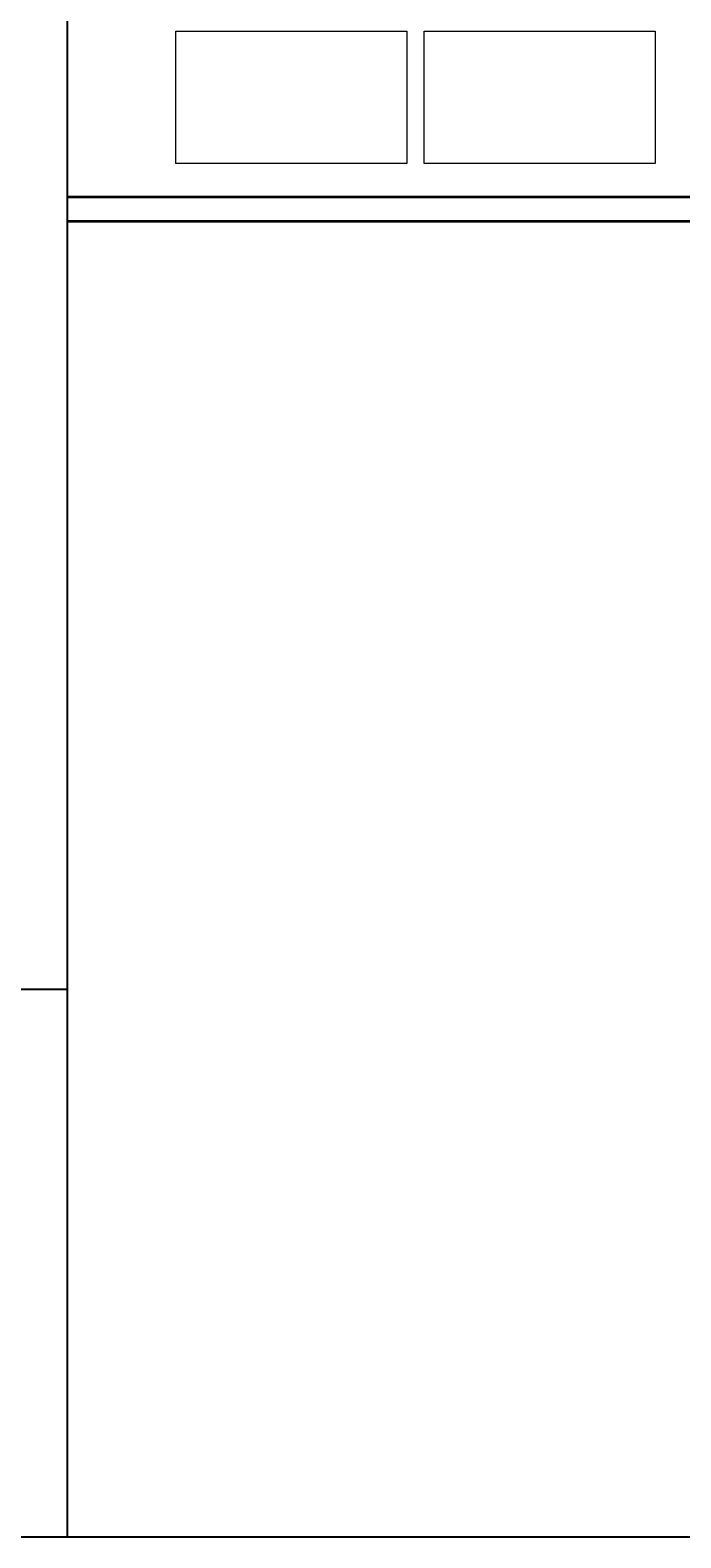
# Model space of a CAD drawing. Units: inches. Extents: x -61 to 1599, y -1316 to 257.
# Tile 155 of 204: x 826 to 989, y -1316 to -939. Entities that reach past the tile are written whole.
import ezdxf

# ---------------------------------------------------------------- set-up
doc = ezdxf.new("R2010")
doc.units = ezdxf.units.IN
doc.header["$MEASUREMENT"] = 0
for name, color, linetype, lineweight in [('A-ANNO-DIMS', 2, 'Continuous', 18), ('A-EQPM', 9, 'Continuous', 18), ('A-FLOR-STRS', 8, 'Continuous', 25), ('WALLS', 4, 'Continuous', 35)]:
    doc.layers.add(name, color=color, linetype=linetype, lineweight=lineweight)
doc.styles.get("Standard").update_dxf_attribs({"font": 'arial.ttf'})
doc.dimstyles.get("Standard").update_dxf_attribs({"dimtxt": 0.18, "dimasz": 0.18, "dimexe": 0.18, "dimexo": 0.0625, "dimgap": 0.09, "dimtad": 0, "dimtih": 1, "dimtoh": 1, "dimdec": 0, "dimzin": 0, "dimdsep": 46, "dimlunit": 3, "dimtxsty": 'Standard', "dimcen": 0.09, "dimadec": 0, "dimazin": 0, "dimtfac": 1, "dimtdec": 0, "dimtofl": 0, "dimtmove": 0, "dimatfit": 3, "dimfxl": 1, "dimtolj": 1, "dimtzin": 0, "dimarcsym": 0})

# ---------------------------------------------------------------- blocks, each defined once
blk = doc.blocks.new('*D689')
at = {"layer": 'A-ANNO-DIMS', "color": 0, "lineweight": -2, "transparency": 16777216}
for p, q in [((992.7, -1211.23), (992.7, -1315.72)), ((544.7, -1216.01), (544.7, -1315.72)), ((544.88, -1315.54), (768.41, -1315.54)), ((992.52, -1315.54), (769, -1315.54))]:
    blk.add_line(p, q, dxfattribs=at)
at = {"layer": 'A-ANNO-DIMS', "color": 0, "transparency": 16777216}
for points in [[(544.88, -1315.51), (544.88, -1315.57), (544.7, -1315.54)], [(992.52, -1315.51), (992.52, -1315.57), (992.7, -1315.54)]]:
    blk.add_solid(points, dxfattribs=at)
at = {"layer": 'DEFPOINTS', "color": 0, "transparency": 16777216}
for p in [(992.7, -1211.17), (544.7, -1215.94), (992.7, -1315.54)]:
    blk.add_point(p, dxfattribs=at)
at = {"layer": 'A-ANNO-DIMS', "color": 0, "transparency": 16777216, "insert": (768.7, -1315.54), "char_height": 0.18, "attachment_point": 5}
blk.add_mtext('\\A1;448', dxfattribs=at)
blk = doc.blocks.new('*D695')
at = {"layer": 'A-ANNO-DIMS', "color": 0, "lineweight": -2, "transparency": 16777216}
for p, q in [((690.7, -1178.86), (690.7, -1315.72)), ((835.7, -1178.86), (835.7, -1315.72)), ((690.88, -1315.54), (762.92, -1315.54)), ((835.52, -1315.54), (763.48, -1315.54))]:
    blk.add_line(p, q, dxfattribs=at)
at = {"layer": 'A-ANNO-DIMS', "color": 0, "transparency": 16777216}
for points in [[(690.88, -1315.51), (690.88, -1315.57), (690.7, -1315.54)], [(835.52, -1315.51), (835.52, -1315.57), (835.7, -1315.54)]]:
    blk.add_solid(points, dxfattribs=at)
at = {"layer": 'DEFPOINTS', "color": 0, "transparency": 16777216}
for p in [(690.7, -1178.79), (835.7, -1178.79), (835.7, -1315.54)]:
    blk.add_point(p, dxfattribs=at)
at = {"layer": 'A-ANNO-DIMS', "color": 0, "transparency": 16777216, "insert": (763.2, -1315.54), "char_height": 0.18, "attachment_point": 5}
blk.add_mtext('\\A1;145', dxfattribs=at)

msp = doc.modelspace()

# ---------------------------------------------------------------- linework, layer by layer
at = {"layer": 'A-EQPM'}
for points in [[(920.4311, -972.7036), (862.8335, -972.7036), (862.8335, -939.7343), (920.4311, -939.7343)], [(982.3846, -972.7036), (924.787, -972.7036), (924.787, -939.7343), (982.3846, -939.7343)]]:
    msp.add_lwpolyline(points, close=True, dxfattribs=at)
at = {"layer": 'A-FLOR-STRS'}
for p in [(835.7028, -891.169), (690.7028, -1178.7933)]:
    msp.add_line(p, (835.7028, -1178.7933), dxfattribs=at)
at = {"layer": 'WALLS'}
for p, q in [((1001.7028, -981.169), (835.7028, -981.169)), ((1001.7028, -987.169), (835.7028, -987.169))]:
    msp.add_line(p, q, dxfattribs=at)

# ---------------------------------------------------------------- dimensions: what is measured, and where the dimension line sits
at = {"layer": 'A-ANNO-DIMS'}
for base, p1, p2, picture, middle in [((835.7028, -1315.5446), (690.7028, -1178.7933), (835.7028, -1178.7933), '*D695', (763.2028, -1315.5446)), ((992.7028, -1315.5446), (544.7028, -1215.9446), (992.7028, -1211.169), '*D689', (768.7028, -1315.5446))]:
    dim = msp.add_linear_dim(base=base, p1=p1, p2=p2, dimstyle='Standard', override={"dimdec": 0, "dimlfac": 1, "dimrnd": 0, "dimzin": 0, "dimdsep": 46, "dimlunit": 2}, dxfattribs=at)
    dim.commit()
    dim.dimension.update_dxf_attribs({"geometry": picture, "text_midpoint": middle})

doc.saveas('drawing.dxf')
